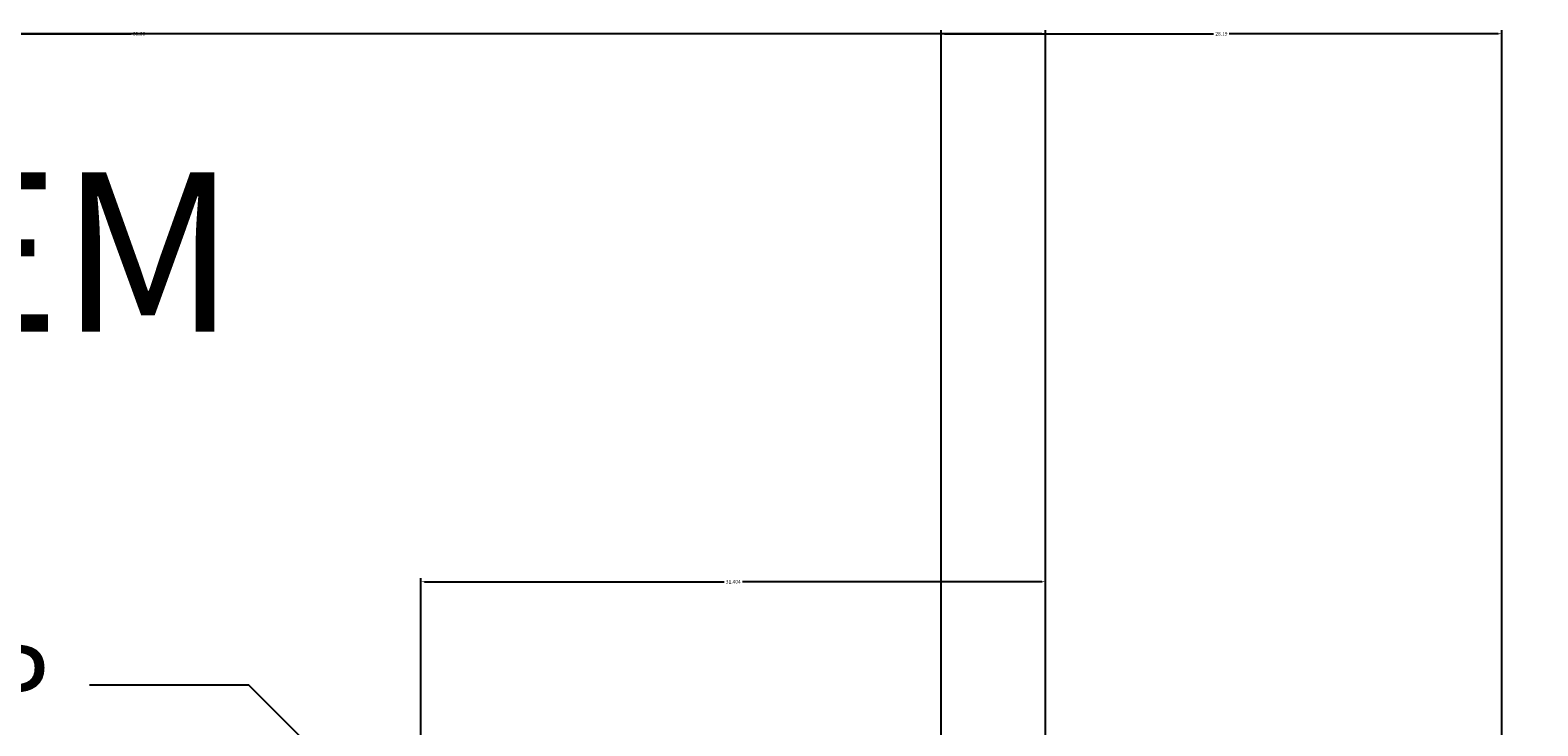
# Model space of a CAD drawing. Units: millimetres. Extents: x -11 to 280, y -4 to 208.
# Tile 55 of 55: x 186 to 262, y 173 to 208. Entities that reach past the tile are written whole.
import ezdxf
from ezdxf import colors
from ezdxf.entities.mleader import LeaderData, LeaderLine
from ezdxf.math import Vec2, Vec3

# ---------------------------------------------------------------- set-up
doc = ezdxf.new("R2010")
doc.units = ezdxf.units.MM
doc.layers.add('M-ANNO-TEXT', color=7, linetype='Continuous', lineweight=18)
doc.layers.add('M-DIMS', color=2, linetype='Continuous', lineweight=18)
doc.styles.get("Standard").update_dxf_attribs({"font": 'arial.ttf'})
doc.dimstyles.get("Standard").update_dxf_attribs({"dimtxt": 0.18, "dimasz": 0.18, "dimexe": 0.18, "dimexo": 0.0625, "dimgap": 0.09, "dimtad": 0, "dimtih": 1, "dimtoh": 1, "dimdec": 4, "dimzin": 0, "dimdsep": 46, "dimtxsty": 'Standard', "dimcen": 0.09, "dimadec": 0, "dimazin": 0, "dimtfac": 1, "dimtdec": 4, "dimtofl": 0, "dimtmove": 0, "dimatfit": 3, "dimfxl": 1, "dimtolj": 1, "dimtzin": 0, "dimarcsym": 0})

# ---------------------------------------------------------------- blocks, each defined once
blk = doc.blocks.new('*D5')
at = {"layer": 'Defpoints', "color": 0, "transparency": 16777216}
for p in [(24.759, 192.645), (-10.087, 11.435), (261.686, 11.435)]:
    blk.add_point(p, dxfattribs=at)
at = {"layer": 'M-DIMS', "color": 0, "lineweight": -2, "transparency": 16777216}
for p, q in [((24.696, 192.645), (-10.267, 192.645)), ((-10.087, 192.465), (-10.087, 102.222)), ((-10.087, 11.615), (-10.087, 101.858)), ((261.624, 11.435), (-10.267, 11.435))]:
    blk.add_line(p, q, dxfattribs=at)
at = {"layer": 'M-DIMS', "color": 0, "transparency": 16777216}
for points in [[(-10.117, 192.465), (-10.057, 192.465), (-10.087, 192.645)], [(-10.117, 11.615), (-10.057, 11.615), (-10.087, 11.435)]]:
    blk.add_solid(points, dxfattribs=at)
at = {"layer": 'M-DIMS', "color": 0, "transparency": 16777216, "insert": (-10.087, 102.04), "char_height": 0.18, "attachment_point": 5}
blk.add_mtext('\\A1;181.2', dxfattribs=at)
blk = doc.blocks.new('*D6')
at = {"layer": 'Defpoints', "color": 0, "transparency": 16777216}
for p in [(236.935, 207.495), (66.388, 179.241), (236.935, 165.103)]:
    blk.add_point(p, dxfattribs=at)
at = {"layer": 'M-DIMS', "color": 0, "lineweight": -2, "transparency": 16777216}
for p, q in [((66.388, 179.304), (66.388, 207.675)), ((66.568, 207.495), (151.206, 207.495)), ((236.755, 207.495), (152.117, 207.495)), ((236.935, 165.166), (236.935, 207.675))]:
    blk.add_line(p, q, dxfattribs=at)
at = {"layer": 'M-DIMS', "color": 0, "transparency": 16777216}
for points in [[(66.568, 207.525), (66.568, 207.465), (66.388, 207.495)], [(236.755, 207.525), (236.755, 207.465), (236.935, 207.495)]]:
    blk.add_solid(points, dxfattribs=at)
at = {"layer": 'M-DIMS', "color": 0, "transparency": 16777216, "insert": (151.661, 207.495), "char_height": 0.18, "attachment_point": 5}
blk.add_mtext('\\A1;170.55', dxfattribs=at)
blk = doc.blocks.new('*D20')
at = {"layer": 'Defpoints', "color": 0, "transparency": 16777216}
for p in [(231.68, 207.495), (151.022, 43.599), (231.68, 43.599)]:
    blk.add_point(p, dxfattribs=at)
at = {"layer": 'M-DIMS', "color": 0, "lineweight": -2, "transparency": 16777216}
for p, q in [((151.022, 43.662), (151.022, 207.675)), ((151.202, 207.495), (190.957, 207.495)), ((231.5, 207.495), (191.745, 207.495)), ((231.68, 43.662), (231.68, 207.675))]:
    blk.add_line(p, q, dxfattribs=at)
at = {"layer": 'M-DIMS', "color": 0, "transparency": 16777216}
for points in [[(151.202, 207.525), (151.202, 207.465), (151.022, 207.495)], [(231.5, 207.525), (231.5, 207.465), (231.68, 207.495)]]:
    blk.add_solid(points, dxfattribs=at)
at = {"layer": 'M-DIMS', "color": 0, "transparency": 16777216, "insert": (191.351, 207.495), "char_height": 0.18, "attachment_point": 5}
blk.add_mtext('\\A1;80.66', dxfattribs=at)
blk = doc.blocks.new('*D22')
at = {"layer": 'Defpoints', "color": 0, "transparency": 16777216}
for p in [(259.871, 207.495), (231.68, 34.723), (259.871, 34.723)]:
    blk.add_point(p, dxfattribs=at)
at = {"layer": 'M-DIMS', "color": 0, "lineweight": -2, "transparency": 16777216}
for p, q in [((231.68, 34.785), (231.68, 207.675)), ((231.86, 207.495), (245.38, 207.495)), ((259.691, 207.495), (246.171, 207.495)), ((259.871, 34.785), (259.871, 207.675))]:
    blk.add_line(p, q, dxfattribs=at)
at = {"layer": 'M-DIMS', "color": 0, "transparency": 16777216}
for points in [[(231.86, 207.525), (231.86, 207.465), (231.68, 207.495)], [(259.691, 207.525), (259.691, 207.465), (259.871, 207.495)]]:
    blk.add_solid(points, dxfattribs=at)
at = {"layer": 'M-DIMS', "color": 0, "transparency": 16777216, "insert": (245.776, 207.495), "char_height": 0.18, "attachment_point": 5}
blk.add_mtext('\\A1;28.19', dxfattribs=at)
blk = doc.blocks.new('*D25')
at = {"layer": 'Defpoints', "color": 0, "transparency": 16777216}
for p in [(236.935, 179.953), (205.531, 165.103), (236.935, 165.103)]:
    blk.add_point(p, dxfattribs=at)
at = {"layer": 'M-DIMS', "color": 0, "lineweight": -2, "transparency": 16777216}
for p, q in [((205.531, 165.166), (205.531, 180.133)), ((205.711, 179.953), (220.77, 179.953)), ((236.755, 179.953), (221.697, 179.953)), ((236.935, 165.166), (236.935, 180.133))]:
    blk.add_line(p, q, dxfattribs=at)
at = {"layer": 'M-DIMS', "color": 0, "transparency": 16777216}
for points in [[(205.711, 179.983), (205.711, 179.923), (205.531, 179.953)], [(236.755, 179.983), (236.755, 179.923), (236.935, 179.953)]]:
    blk.add_solid(points, dxfattribs=at)
at = {"layer": 'M-DIMS', "color": 0, "transparency": 16777216, "insert": (221.233, 179.953), "char_height": 0.18, "attachment_point": 5}
blk.add_mtext('\\A1;31.404', dxfattribs=at)

msp = doc.modelspace()

# ---------------------------------------------------------------- texts
at = {"layer": 'M-ANNO-TEXT', "insert": (94.3946, 200.5299), "char_height": 8, "attachment_point": 1}
msp.add_mtext_dynamic_manual_height_columns('HYDRAULIC SYSTEM ', width=219.105197, gutter_width=12.5, heights=[0], dxfattribs=at)

# ---------------------------------------------------------------- dimensions: what is measured, and where the dimension line sits
at = {"layer": 'M-DIMS'}
for base, p1, p2, override, picture, middle in [((236.9353, 207.495), (66.3875, 179.2412), (236.9353, 165.103), {"dimdec": 2, "dimlfac": 1, "dimrnd": 0, "dimzin": 0, "dimdsep": 46, "dimlunit": 2}, '*D6', (151.6614, 207.495)), ((231.6803, 207.495), (151.0217, 43.5991), (231.6803, 43.5991), {"dimdec": 2, "dimlfac": 1, "dimrnd": 0, "dimzin": 0, "dimdsep": 46, "dimlunit": 2}, '*D20', (191.351, 207.495)), ((259.871, 207.495), (231.6803, 34.7226), (259.871, 34.7226), {"dimdec": 2, "dimlfac": 1, "dimrnd": 0, "dimzin": 0, "dimdsep": 46, "dimlunit": 2}, '*D22', (245.7757, 207.495)), ((236.9353, 179.953), (205.5315, 165.103), (236.9353, 165.103), {"dimdec": 3, "dimlfac": 1, "dimrnd": 0, "dimzin": 0, "dimdsep": 46, "dimlunit": 2}, '*D25', (221.2334, 179.953))]:
    dim = msp.add_linear_dim(base=base, p1=p1, p2=p2, dimstyle='Standard', override=override, dxfattribs=at)
    dim.commit()
    dim.dimension.update_dxf_attribs({"geometry": picture, "text_midpoint": middle})
dim = msp.add_linear_dim(base=(-10.0865, 11.4346), p1=(24.7588, 192.645), p2=(261.6863, 11.4346), angle=90, dimstyle='Standard', override={"dimdec": 1, "dimlfac": 1, "dimrnd": 0, "dimzin": 0, "dimdsep": 46, "dimlunit": 2}, dxfattribs=at)
dim.commit()
dim.dimension.update_dxf_attribs({"geometry": '*D5', "text_midpoint": (-10.0865, 102.0398)})

# ---------------------------------------------------------------- leaders
at = {"layer": 'M-ANNO-TEXT'}
ml = msp.add_multileader_mtext('Standard', dxfattribs=at)
ml.set_content('HAND PUMP', color=256)
ml.set_leader_properties()
ml.build(insert=Vec2(0, 0))
ctx = ml.context
ctx.base_point, ctx.plane_origin = Vec3(152.0312, 174.7629), Vec3(205.5315, 166.103)
ctx.text_align_type = 2
notes = []
notes.append((ctx, [(0, (1, 1, 0), (196.8716, 174.7629), (-1, 0), 8, [(0, [(205.5315, 166.103)], 0, [])])]))
ctx.mtext.insert, ctx.mtext.alignment, ctx.mtext.flow_direction = Vec3(186.8716, 176.7971), 3, 5
for ctx, leaders in notes:
    for number, flags, end, landing, length, lines in leaders:
        leader = LeaderData()
        leader.index, (leader.has_last_leader_line, leader.has_dogleg_vector, leader.attachment_direction) = number, flags
        leader.last_leader_point, leader.dogleg_vector, leader.dogleg_length = Vec3(end), Vec3(landing), length
        for number, points, colour, breaks in lines:
            line = LeaderLine()
            line.index, line.vertices, line.color, line.breaks = number, Vec3.list(points), colors.encode_raw_color(colour), breaks
            leader.lines.append(line)
        ctx.leaders.append(leader)

doc.saveas('drawing.dxf')
